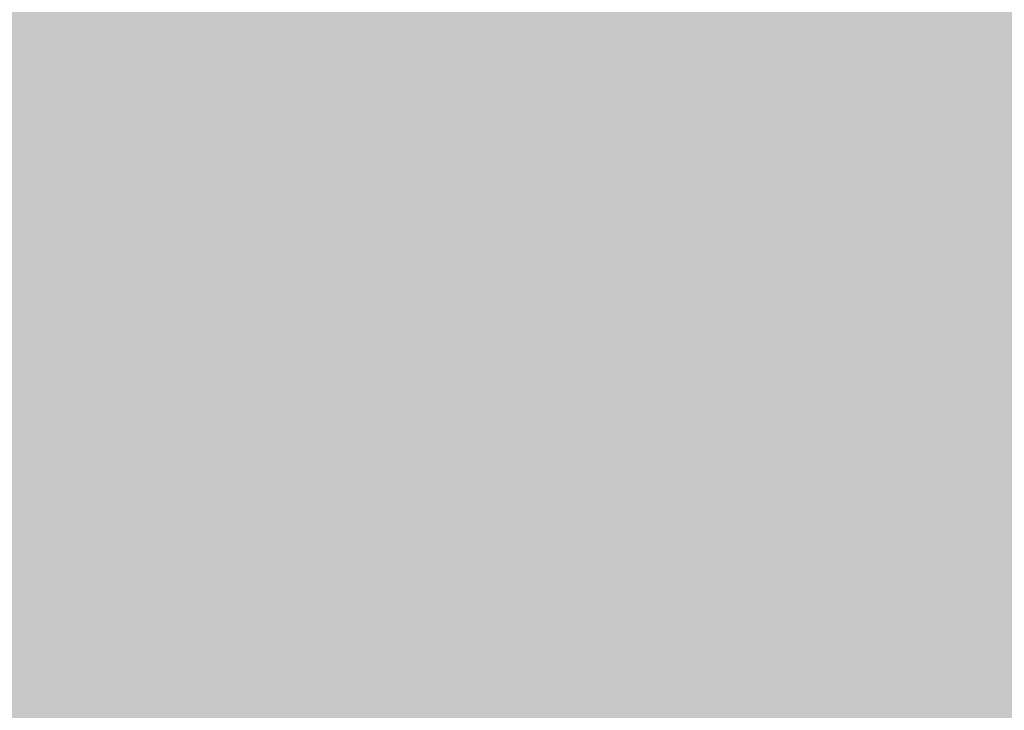
# Model space of a CAD drawing. Units: inches. Extents: x 2091 to 2899, y 967 to 2217.
# Tile 204 of 256: x 2203.18039 to 2203.25707, y 1152.30086 to 1152.35465. Entities that reach past the tile are written whole.
import ezdxf

# ---------------------------------------------------------------- set-up
doc = ezdxf.new("R2010")
doc.units = ezdxf.units.IN
doc.layers.add('A-WALL-PATT', color=141, linetype='Continuous', lineweight=13, true_color=0xadddf7)

msp = doc.modelspace()

# ---------------------------------------------------------------- hatches: boundary and pattern name
at = {"layer": 'A-WALL-PATT'}
h = msp.add_hatch(color=256, dxfattribs=at)
h.dxf.hatch_style = 1
h.paths.add_polyline_path([(2803.143603, 2050.919059), (2203.143603, 2050.919059), (2203.143603, 1090.919059), (2803.143603, 1090.919059)])
h.paths.add_polyline_path([(2635.79885, 1147.540465), (2674.524052, 1147.540465, 0.376086), (2678.529665, 1152.880202), (2678.529665, 1159.556473, 0.333335), (2674.524319, 1163.561846), (2674.524319, 1163.56185), (2674.524319, 1192.93439), (2635.805971, 1192.93439), (2597.087622, 1192.93439), (2597.087622, 1163.561846, 0.333335), (2593.082276, 1159.556473), (2593.082276, 1152.880202, 0.376086), (2597.087889, 1147.540465)], flags=0)
h.paths.add_polyline_path([(2436.010433, 1278.240778, 0.000483), (2435.952643, 1278.215027, -0.001328), (2435.935625, 1278.111693, -0.001711), (2436.11644, 1278.040758, 0.002185)], flags=0)
h.paths.add_polyline_path([(2794.143603, 1143.419059), (2794.143603, 1347.419059), (2543.370171, 1347.419059), (2543.370171, 1351.919059), (2794.143603, 1351.919059), (2794.143603, 1392.713555), (2793.947398, 1392.713555), (2793.947398, 1473.5369), (2794.143603, 1473.5369), (2794.143603, 1531.919059), (2650.143603, 1531.919059), (2650.143603, 1536.419059), (2794.143603, 1536.419059), (2794.143603, 1692.419059), (2609.375609, 1692.419059), (2609.375609, 1644.419059), (2604.875609, 1644.419059), (2604.875609, 1744.919059), (2609.375609, 1744.919059), (2609.375609, 1696.919059), (2794.143603, 1696.919059), (2794.143603, 1780.919059), (2609.643603, 1780.919059), (2493.875609, 1780.919059), (2493.875609, 1785.419059), (2609.643603, 1785.419059), (2794.143603, 1785.419059), (2794.143603, 1847.938821), (2793.951222, 1847.938821), (2793.951222, 1928.762166), (2794.143603, 1928.762166), (2794.143603, 1941.419059), (2614.143603, 1941.419059), (2614.143603, 1821.419059), (2609.643603, 1821.419059), (2609.643603, 1941.419059), (2392.143603, 1941.419059), (2392.143603, 1819.919059), (2387.643603, 1819.919059), (2387.643603, 1941.419059), (2212.143603, 1941.419059), (2212.143603, 1783.919059), (2392.143603, 1783.919059), (2392.143603, 1780.919059), (2212.143603, 1780.919059), (2212.143603, 1629.419059), (2387.643603, 1629.419059), (2387.643603, 1744.919059), (2392.143603, 1744.919059), (2392.143603, 1627.919059), (2317.143603, 1627.919059), (2317.143603, 1551.419059), (2317.143603, 1536.419059), (2459.383591, 1536.419059), (2459.383591, 1602.39648), (2463.883591, 1602.39648), (2463.883591, 1531.919059), (2456.643603, 1531.919059), (2456.643603, 1529.919059), (2452.143603, 1529.919059), (2452.143603, 1531.919059), (2312.643603, 1531.919059), (2312.643603, 1551.419059), (2306.143603, 1551.419059), (2306.143603, 1555.919059), (2308.143603, 1555.919059), (2308.143603, 1551.419059), (2312.643603, 1551.419059), (2312.643603, 1627.919059), (2212.143603, 1627.919059), (2212.143603, 1555.919059), (2270.143603, 1555.919059), (2270.143603, 1551.419059), (2212.143603, 1551.419059), (2212.143603, 1351.919059), (2272.143603, 1351.919059), (2272.143603, 1347.419059), (2212.143603, 1347.419059), (2212.143603, 1275.419059), (2308.143603, 1275.419059), (2308.143603, 1351.919059), (2452.143603, 1351.919059), (2452.143603, 1493.919059), (2456.643603, 1493.919059), (2456.643603, 1347.419059), (2312.643603, 1347.419059), (2312.643603, 1270.919059), (2212.143603, 1270.919059), (2212.143603, 1099.919059), (2281.237523, 1099.919059), (2282.871041, 1110.913803), (2282.008341, 1116.996603), (2278.557741, 1121.420403), (2268.205641, 1128.056203), (2272.087641, 1128.056203), (2273.812941, 1131.927003), (2279.420341, 1134.691903), (2285.027841, 1135.244903), (2287.615841, 1137.456803), (2288.047141, 1138.009803), (2289.341141, 1140.774703), (2291.066541, 1139.668703), (2292.360541, 1135.244903), (2295.379841, 1136.903803), (2296.242541, 1135.797903), (2297.105241, 1133.033003), (2300.124641, 1138.009803), (2303.143941, 1138.009803), (2304.437941, 1135.797903), (2303.143941, 1133.586003), (2306.594641, 1134.691903), (2307.888741, 1133.033003), (2310.908041, 1135.244903), (2313.927441, 1134.138903), (2315.62686, 1132.427102), (2308.320041, 1117.549603), (2290.203841, 1109.807903), (2288.909841, 1103.172103), (2289.272309, 1099.919059), (2434.918227, 1099.919059), (2431.593227, 1124.788059), (2429.930227, 1169.553059), (2430.927185, 1240.519694), (2435.658926, 1238.186126), (2437.135227, 1196.554059), (2438.798227, 1143.973059), (2442.678227, 1111.998059), (2446.558227, 1099.919059), (2794.143603, 1099.919059), (2794.143603, 1138.919059), (2548.032447, 1138.919059), (2548.032447, 1143.419059), (2548.032447, 1148.819059), (2546.668457, 1148.031559), (2528.685692, 1179.178622, 0.256256), (2512.032447, 1148.819059), (2512.032447, 1143.419059), (2512.032447, 1138.919059), (2507.532447, 1138.919059), (2507.532447, 1143.419059), (2507.532447, 1148.819059, 0.256256), (2490.879202, 1179.178622), (2472.896437, 1148.031559), (2471.532447, 1148.819059), (2471.532447, 1143.419059), (2467.032447, 1143.419059), (2467.032447, 1269.945786, 0.039061), (2460.909987, 1273.580059), (2467.032447, 1273.580059), (2467.032447, 1286.325364, 0.014511), (2465.216194, 1286.761905), (2467.032447, 1287.052576), (2467.032447, 1323.419059), (2471.532447, 1323.419059), (2471.532447, 1148.819059), (2489.532447, 1179.995973), (2490.896437, 1179.208473), (2490.879202, 1179.178622, -0.256256), (2507.532447, 1148.819059), (2507.532447, 1143.419059), (2512.032447, 1143.419059), (2512.032447, 1148.819059, -0.256256), (2528.685692, 1179.178622), (2528.668457, 1179.208473), (2530.032447, 1179.995973), (2548.032447, 1148.819059), (2548.032447, 1143.419059)], flags=16)
h.paths.add_polyline_path([(2607.768546, 1200.945083), (2607.768546, 1265.030625), (2597.087622, 1281.052011), (2619.784585, 1281.052011), (2627.795278, 1337.12686), (2635.79885, 1337.12686), (2643.816663, 1337.12686), (2651.827356, 1281.052011), (2674.524319, 1281.052011), (2663.843395, 1265.030625), (2663.843395, 1200.945083), (2635.805971, 1200.945083)], flags=0)
edge = h.paths.add_edge_path(flags=0)
edge.add_ellipse((13303.896215, 1272.998725), major_axis=(-10595.31304, 0.000001), ratio=0.842303870086, start_angle=0.6282372191, end_angle=0.6465540999, ccw=False)
edge.add_ellipse((2711.70045, 1156.852678), major_axis=(2.219769, 0), ratio=0.84230387, start_angle=111.535244, end_angle=180.628237, ccw=False)
edge.add_ellipse((13303.156292, 1272.998725), major_axis=(-10593.026306, 0), ratio=0.842303869544, start_angle=0.5282714718, end_angle=0.6465540971, ccw=False)
edge.add_line((2710.764596, 1175.333295), (2710.129986, 1175.333295))
edge.add_ellipse((2710.129986, 1176.579775), major_axis=(1.479846, 0), ratio=0.84230387, start_angle=180, end_angle=270, ccw=False)
edge.add_line((2708.65014, 1176.579775), (2708.65014, 1200.782914))
edge.add_ellipse((2710.129986, 1200.782914), major_axis=(1.479846, 0), ratio=0.84230387, start_angle=90, end_angle=180, ccw=False)
edge.add_line((2710.129986, 1202.029394), (2710.465075, 1202.029394))
edge.add_ellipse((13303.156292, 1272.998725), major_axis=(-10593.026306, 0), ratio=0.842303869544, start_angle=-0.0902290886, end_angle=0.3838667788, ccw=False)
edge.add_ellipse((2710.129986, 1290.927031), major_axis=(-1.479846, 0), ratio=0.84230387, start_angle=0, end_angle=90, ccw=False)
edge.add_line((2708.65014, 1290.927031), (2708.65014, 1315.13017))
edge.add_ellipse((2710.129986, 1315.13017), major_axis=(-1.479846, 0), ratio=0.84230387, start_angle=-90, end_angle=0, ccw=False)
edge.add_line((2710.129986, 1316.37665), (2710.706314, 1316.37665))
edge.add_ellipse((3238.40172, 1296.289566), major_axis=(528.234, 0), ratio=0.8423038695, start_angle=176.34957241, end_angle=177.82004969, ccw=False)
edge.add_ellipse((2775.063043, 1071.450696), major_axis=(313.307761, 0), ratio=0.8423038695, start_angle=102.12596555, end_angle=103.78052899, ccw=False)
edge.add_ellipse((2775.063043, 1078.305698), major_axis=(-305.302891, 0), ratio=0.8423038695, start_angle=-79.790461, end_angle=-77.55537271, ccw=False)
edge.add_ellipse((2695.141767, 1541.975383), major_axis=(-250.960216, 0), ratio=0.8423038695, start_angle=99.25656601, end_angle=102.55493264)
edge.add_line((2741.410326, 1334.214255), (2747.132545, 1337.378477))
edge.add_ellipse((2747.538616, 1336.857478), major_axis=(-0.739923, 0), ratio=0.8423039, start_angle=270, end_angle=307.93313, ccw=False)
edge.add_ellipse((2747.538616, 1336.857478), major_axis=(-0.739923, 0), ratio=0.8423039, start_angle=232.06687, end_angle=270, ccw=False)
edge.add_line((2747.944687, 1337.378477), (2753.666906, 1334.214255))
edge.add_ellipse((2799.935466, 1541.975383), major_axis=(250.960216, 0), ratio=0.8423038695, start_angle=257.44506736, end_angle=260.74343399)
edge.add_ellipse((2720.014189, 1078.305698), major_axis=(305.302891, 0), ratio=0.8423038695, start_angle=77.55537271, end_angle=79.790461, ccw=False)
edge.add_ellipse((2720.014189, 1071.450696), major_axis=(-313.307761, 0), ratio=0.8423038695, start_angle=256.21947101, end_angle=257.87403445, ccw=False)
edge.add_ellipse((2256.675512, 1296.289566), major_axis=(-528.234, 0), ratio=0.8423038695, start_angle=182.17995031, end_angle=183.65042759, ccw=False)
edge.add_line((2784.370918, 1316.37665), (2784.947247, 1316.37665))
edge.add_ellipse((2784.947247, 1315.13017), major_axis=(1.479846, 0), ratio=0.84230387, start_angle=0, end_angle=90, ccw=False)
edge.add_line((2786.427093, 1315.13017), (2786.427093, 1290.927031))
edge.add_ellipse((2784.947247, 1290.927031), major_axis=(1.479846, 0), ratio=0.84230387, start_angle=270, end_angle=360, ccw=False)
edge.add_ellipse((-7808.07906, 1272.998725), major_axis=(10593.026306, 0), ratio=0.842303869544, start_angle=-0.3838667788, end_angle=0.0902290886, ccw=False)
edge.add_line((2784.612157, 1202.029394), (2784.947247, 1202.029394))
edge.add_ellipse((2784.947247, 1200.782914), major_axis=(1.479846, 0), ratio=0.84230387, start_angle=0, end_angle=90, ccw=False)
edge.add_line((2786.427093, 1200.782914), (2786.427093, 1176.579775))
edge.add_ellipse((2784.947247, 1176.579775), major_axis=(-1.479846, 0), ratio=0.84230387, start_angle=90, end_angle=180, ccw=False)
edge.add_line((2784.947247, 1175.333295), (2784.312636, 1175.333295))
edge.add_ellipse((-7808.07906, 1272.998725), major_axis=(10593.026306, 0), ratio=0.842303869544, start_angle=-0.6186431963, end_angle=-0.5282714718, ccw=False)
edge.add_ellipse((2783.376783, 1156.852678), major_axis=(-2.219769, 0), ratio=0.84230387, start_angle=179.371763, end_angle=248.464757, ccw=False)
edge.add_ellipse((-7808.818983, 1272.998725), major_axis=(-10595.31304, 0.000004), ratio=0.842303865762, start_angle=179.3534459226, end_angle=179.3717628034, ccw=False)
edge.add_ellipse((2780.297303, 1153.500793), major_axis=(-5.246426, 0), ratio=0.84230387, start_angle=90, end_angle=179.353446, ccw=False)
edge.add_line((2780.297303, 1149.081708), (2714.77993, 1149.081708))
edge.add_ellipse((2714.77993, 1153.500793), major_axis=(5.246426, 0), ratio=0.84230387, start_angle=180.646554, end_angle=270, ccw=False)
edge = h.paths.add_edge_path(flags=0)
edge.add_line((2718.187367, 1151.007833), (2718.187367, 1170.472364))
edge.add_ellipse((2721.14706, 1170.472364), major_axis=(-2.959692, 0), ratio=0.84230387, start_angle=-90, end_angle=0, ccw=False)
edge.add_line((2721.14706, 1172.965324), (2773.930173, 1172.965324))
edge.add_ellipse((2773.930173, 1170.472364), major_axis=(-2.959692, 0), ratio=0.84230387, start_angle=180, end_angle=270, ccw=False)
edge.add_line((2776.889865, 1170.472364), (2776.889865, 1151.007833))
edge.add_line((2776.889865, 1151.007833), (2718.187367, 1151.007833))
edge = h.paths.add_edge_path(flags=0)
edge.add_line((2718.187367, 1180.23415), (2718.187367, 1199.057834))
edge.add_ellipse((2747.538616, 1320.39864), major_axis=(147.017924, 0), ratio=0.8423038695, start_angle=256.40186531, end_angle=283.59813469)
edge.add_line((2776.889865, 1199.057834), (2776.889865, 1180.23415))
edge.add_ellipse((2747.538616, 1301.574956), major_axis=(147.017924, 0), ratio=0.8423038695, start_angle=256.40186531, end_angle=283.59813469, ccw=False)
edge = h.paths.add_edge_path(flags=0)
edge.add_ellipse((13303.156292, 1272.998725), major_axis=(-10591.54646, 0), ratio=0.842303869555, start_angle=0.0555943135, end_angle=0.3777641939, ccw=False)
edge.add_line((2711.616859, 1262.72171), (2715.667408, 1249.495396))
edge.add_ellipse((6413.891963, 1241.691919), major_axis=(-3698.236159, 0), ratio=0.84230386955, start_angle=-0.120897369, end_angle=0.364076349)
edge.add_line((2715.761038, 1218.192455), (2711.934307, 1203.167361))
edge = h.paths.add_edge_path(flags=0)
edge.add_line((2718.187367, 1251.074566), (2716.002485, 1267.450435))
edge.add_ellipse((2742.151175, 1202.18954), major_axis=(81.772585, 0), ratio=0.84230387, start_angle=94.27742096, end_angle=111.8349538, ccw=False)
edge.add_line((2737.009748, 1270.930626), (2758.067484, 1270.930626))
edge.add_ellipse((2752.926058, 1202.18954), major_axis=(81.772585, 0), ratio=0.84230387, start_angle=68.1650462, end_angle=85.72257904, ccw=False)
edge.add_line((2779.074747, 1267.450435), (2776.889865, 1251.074566))
edge.add_ellipse((2750.338059, 1187.885356), major_axis=(79.579664, 0), ratio=0.84230387, start_angle=67.20808512, end_angle=85.1299304)
edge.add_line((2756.034656, 1254.743656), (2739.042576, 1254.743656))
edge.add_ellipse((2744.739174, 1187.885356), major_axis=(79.579664, 0), ratio=0.84230387, start_angle=94.8700696, end_angle=112.79191488)
edge = h.paths.add_edge_path(flags=0)
edge.add_line((2783.142926, 1203.167361), (2779.316194, 1218.192455))
edge.add_ellipse((-918.81473, 1241.691919), major_axis=(3698.236159, 0), ratio=0.84230386955, start_angle=-0.364076349, end_angle=0.120897369)
edge.add_line((2779.409825, 1249.495396), (2783.460373, 1262.72171))
edge.add_ellipse((-7808.07906, 1272.998725), major_axis=(-10591.54646, 0), ratio=0.84230386954, start_angle=179.6222358061, end_angle=179.9444056865, ccw=False)
edge = h.paths.add_edge_path(flags=0)
edge.add_ellipse((2734.200892, 1286.69044), major_axis=(-0.356609, 6.340078), ratio=0.60383358, start_angle=89.0020143, end_angle=253.657408, ccw=False)
edge.add_line((2730.369001, 1286.541806), (2730.369001, 1301.35198))
edge.add_line((2730.369001, 1301.35198), (2735.913311, 1305.214803))
edge.add_ellipse((2736.384917, 1304.734561), major_axis=(0.739923, 0), ratio=0.8423039, start_angle=90, end_angle=134.480211, ccw=False)
edge.add_line((2736.384917, 1305.357801), (2738.032783, 1305.357801))
edge.add_line((2738.032783, 1305.357801), (2738.032783, 1307.707927))
edge.add_ellipse((2794.201642, 1307.707927), major_axis=(56.168859, 0), ratio=0.84230387, start_angle=150.5614304, end_angle=180, ccw=False)
edge.add_ellipse((2700.875591, 1307.707927), major_axis=(-56.168859, 0), ratio=0.84230387, start_angle=180, end_angle=209.4385696, ccw=False)
edge.add_line((2757.04445, 1307.707927), (2757.04445, 1305.357801))
edge.add_line((2757.04445, 1305.357801), (2758.692316, 1305.357801))
edge.add_ellipse((2758.692316, 1304.734561), major_axis=(-0.739923, 0), ratio=0.8423039, start_angle=225.519789, end_angle=270, ccw=False)
edge.add_line((2759.163922, 1305.214803), (2764.708231, 1301.35198))
edge.add_line((2764.708231, 1301.35198), (2764.708231, 1286.541806))
edge.add_ellipse((2760.87634, 1286.69044), major_axis=(0.356609, 6.340078), ratio=0.60383358, start_angle=106.342592, end_angle=270.9979857, ccw=False)
edge.add_line((2757.04445, 1285.79709), (2757.04445, 1307.707927))
edge.add_ellipse((2700.875591, 1307.707927), major_axis=(-56.168859, 0), ratio=0.84230387, start_angle=180, end_angle=209.4385696)
edge.add_ellipse((2794.201642, 1307.707927), major_axis=(56.168859, 0), ratio=0.84230387, start_angle=150.5614304, end_angle=180)
edge.add_line((2738.032783, 1307.707927), (2738.032783, 1285.79709))
h.paths.add_polyline_path([(2417.812273, 1104.449704), (2413.492273, 1102.529704), (2410.612273, 1103.969704), (2409.172273, 1106.369704), (2407.252273, 1107.329704), (2406.292273, 1109.729704), (2405.332273, 1114.049704), (2405.332273, 1117.889704), (2406.292273, 1120.129704), (2407.252273, 1119.809704), (2408.848322, 1118.327658), (2410.173945, 1119.42417), (2410.211273, 1120.405704), (2411.040731, 1121.419054), (2410.699273, 1119.858704), (2410.173945, 1119.42417), (2410.088452, 1117.176109), (2411.132836, 1116.206324), (2413.972273, 1119.329704), (2416.852273, 1120.769704), (2416.869721, 1120.798784), (2417.035071, 1119.405116), (2417.896213, 1118.143384), (2418.292273, 1118.369704), (2419.544447, 1120.039269), (2419.360915, 1118.387487), (2419.032108, 1119.356151), (2418.398939, 1118.511926), (2419.252273, 1114.529704), (2418.794091, 1107.198795)], flags=0)
h.paths.add_polyline_path([(2508.870171, 1347.419059), (2508.370171, 1347.419059), (2508.370171, 1351.919059), (2508.870171, 1351.919059)], flags=0)
h.paths.add_polyline_path([(2473.370171, 1347.419059), (2472.370171, 1347.419059), (2467.870171, 1347.419059), (2467.870171, 1455.419059), (2472.370171, 1455.419059), (2472.370171, 1352.419059), (2473.370171, 1352.419059)], flags=0)
h.paths.add_polyline_path([(2352.106244, 1217.446197), (2349.226244, 1218.886197), (2347.786244, 1221.286197), (2345.866244, 1222.246197), (2344.906244, 1224.646197), (2343.946244, 1228.966197), (2343.946244, 1232.806197), (2344.906244, 1235.046197), (2345.866244, 1234.726197), (2347.462293, 1233.244152), (2348.787916, 1234.340663), (2348.825244, 1235.322197), (2349.654702, 1236.335547), (2349.313244, 1234.775197), (2348.787916, 1234.340663), (2348.702423, 1232.092603), (2349.746807, 1231.122817), (2352.586244, 1234.246197), (2355.466244, 1235.686197), (2355.483692, 1235.715277), (2355.649043, 1234.321609), (2356.510185, 1233.059877), (2356.906244, 1233.286197), (2358.158418, 1234.955762), (2357.974887, 1233.30398), (2357.646079, 1234.272644), (2357.012911, 1233.428419), (2357.866244, 1229.446197), (2357.408062, 1222.115288), (2356.426244, 1219.366197)], flags=0)
h.paths.add_polyline_path([(2348.2968, 1112.22442), (2347.0138, 1112.31042), (2345.5298, 1114.12742), (2345.7318, 1115.85842), (2346.8118, 1116.98242), (2346.8118, 1114.64642), (2345.8668, 1114.21442), (2346.8798, 1114.30042)], flags=0)
h.paths.add_polyline_path([(2347.0138, 1110.92642), (2346.2718, 1110.49342), (2346.6098, 1111.18642)], flags=0)
h.paths.add_polyline_path([(2345.8668, 1118.19442), (2345.5298, 1117.32942), (2343.7078, 1118.02142), (2344.3828, 1118.62642)], flags=0)
h.paths.add_polyline_path([(2346.6768, 1109.28242), (2346.0698, 1108.07142), (2345.8668, 1110.06142)], flags=0)
h.paths.add_polyline_path([(2345.0568, 1119.75142), (2343.6398, 1119.75142), (2343.9778, 1121.13542)], flags=0)
h.paths.add_polyline_path([(2345.2598, 1116.55042), (2345.1248, 1115.85842), (2344.9218, 1115.68542), (2344.7198, 1116.37742)], flags=0)
h.paths.add_polyline_path([(2345.6648, 1112.31042), (2345.4618, 1111.53242), (2344.0448, 1111.96442), (2344.6518, 1112.57042)], flags=0)
h.paths.add_polyline_path([(2345.1918, 1113.34942), (2344.4498, 1113.86842), (2344.7198, 1114.38742)], flags=0)
h.paths.add_polyline_path([(2344.6518, 1116.80942), (2344.1798, 1115.68542), (2344.6518, 1115.33942), (2343.9098, 1114.90642), (2343.0328, 1115.94442), (2343.6398, 1116.46342)], flags=0)
h.paths.add_polyline_path([(2345.8668, 1106.68642), (2344.9898, 1105.56242), (2344.5168, 1106.60042)], flags=0)
h.paths.add_polyline_path([(2344.8548, 1110.06142), (2344.5168, 1109.28242), (2344.1128, 1109.71542)], flags=0)
h.paths.add_polyline_path([(2344.0448, 1113.52242), (2343.4378, 1113.08942), (2342.7628, 1113.95442)], flags=0)
h.paths.add_polyline_path([(2344.3148, 1111.01242), (2342.9648, 1110.32042), (2342.9648, 1111.09942)], flags=0)
h.paths.add_polyline_path([(2345.1248, 1104.69742), (2344.5848, 1103.74542), (2344.4498, 1104.26442)], flags=0)
h.paths.add_polyline_path([(2342.8298, 1121.22242), (2341.7498, 1120.53042), (2340.5358, 1121.04942), (2340.1308, 1121.82842), (2340.6708, 1122.95242), (2341.1428, 1121.82842), (2341.6148, 1122.00142)], flags=0)
h.paths.add_polyline_path([(2342.9648, 1119.75142), (2343.0328, 1118.45342), (2342.0878, 1118.02142), (2342.0198, 1119.49142)], flags=0)
h.paths.add_polyline_path([(2342.6948, 1116.89642), (2341.9528, 1116.63642), (2342.0198, 1117.32942)], flags=0)
h.paths.add_polyline_path([(2343.0328, 1112.22442), (2342.0198, 1111.79142), (2341.5478, 1112.22442), (2342.3578, 1113.34942)], flags=0)
h.paths.add_polyline_path([(2343.7748, 1104.43742), (2342.6278, 1102.88042), (2342.6948, 1104.61042), (2343.4378, 1105.12942)], flags=0)
h.paths.add_polyline_path([(2342.0198, 1115.07942), (2340.8058, 1115.51242), (2340.9408, 1116.37742)], flags=0)
h.paths.add_polyline_path([(2341.4808, 1120.09742), (2341.4808, 1119.40542), (2341.0758, 1119.57842), (2341.1428, 1120.09742)], flags=0)
h.paths.add_polyline_path([(2341.8178, 1114.47342), (2340.9408, 1113.08942), (2340.8058, 1114.56042)], flags=0)
h.paths.add_polyline_path([(2341.1428, 1118.54042), (2340.9408, 1116.98242), (2339.0508, 1117.67542), (2339.0508, 1118.62642)], flags=0)
h.paths.add_polyline_path([(2342.6948, 1101.66842), (2341.9528, 1101.84142), (2342.5598, 1102.36142)], flags=0)
h.paths.add_polyline_path([(2340.3328, 1119.66542), (2338.4438, 1119.57842), (2337.9038, 1120.35742), (2339.6578, 1120.61642)], flags=0)
h.paths.add_polyline_path([(2340.3328, 1115.33942), (2340.0628, 1113.69542), (2339.3878, 1115.33942)], flags=0)
h.paths.add_polyline_path([(2341.8178, 1103.83142), (2341.5478, 1102.88042), (2341.1428, 1103.65842)], flags=0)
h.paths.add_polyline_path([(2339.0508, 1122.86642), (2337.2958, 1121.82842), (2337.0938, 1123.12542), (2337.7688, 1123.81842)], flags=0)
h.paths.add_polyline_path([(2339.1178, 1121.74142), (2338.8478, 1121.22242), (2338.1738, 1121.04942), (2338.3758, 1121.56842)], flags=0)
h.paths.add_polyline_path([(2339.1858, 1119.31942), (2338.6458, 1118.71342), (2338.2408, 1118.10742), (2338.2408, 1118.88642)], flags=0)
h.paths.add_polyline_path([(2341.1428, 1101.92842), (2340.6028, 1101.23642), (2340.0628, 1101.84142), (2340.6028, 1102.36142)], flags=0)
h.paths.add_polyline_path([(2337.6338, 1117.76142), (2336.6208, 1118.28042), (2337.2958, 1118.97242)], flags=0)
h.paths.add_polyline_path([(2336.8238, 1119.57842), (2334.7988, 1118.97242), (2335.2038, 1120.35742), (2336.5538, 1120.87642)], flags=0)
h.paths.add_polyline_path([(2339.1178, 1100.45742), (2337.3638, 1100.54342), (2336.7558, 1101.23642)], flags=0)
h.paths.add_polyline_path([(2336.3508, 1122.43342), (2336.0138, 1121.91442), (2334.9338, 1122.43342), (2334.5288, 1123.47142), (2335.7438, 1122.77942)], flags=0)
h.paths.add_polyline_path([(2334.7318, 1120.87642), (2334.2588, 1120.35742), (2334.0568, 1120.78942), (2334.5968, 1121.30842)], flags=0)
h.paths.add_polyline_path([(2334.4618, 1122.17442), (2332.5718, 1121.30842), (2331.3568, 1122.17442), (2332.0998, 1122.86642)], flags=0)
h.paths.add_polyline_path([(2334.2588, 1118.54042), (2333.3818, 1118.45342), (2333.6518, 1119.31942)], flags=0)
h.paths.add_polyline_path([(2335.5418, 1102.27442), (2334.1918, 1102.62042), (2335.2718, 1103.31242)], flags=0)
h.paths.add_polyline_path([(2332.7068, 1119.66542), (2331.6948, 1120.44342), (2332.5048, 1120.78942)], flags=0)
h.paths.add_polyline_path([(2334.7318, 1101.14942), (2333.5168, 1101.58242), (2333.9888, 1101.75542)], flags=0)
h.paths.add_polyline_path([(2332.6398, 1116.63642), (2331.0868, 1116.29042), (2331.9648, 1118.19442)], flags=0)
h.paths.add_polyline_path([(2330.7498, 1121.56842), (2330.2768, 1120.27042), (2328.5228, 1119.31942), (2328.9948, 1121.04942)], flags=0)
h.paths.add_polyline_path([(2330.7498, 1118.62642), (2330.0078, 1117.50242), (2329.8728, 1118.02142)], flags=0)
h.paths.add_polyline_path([(2332.0998, 1102.36142), (2330.5468, 1102.01442), (2331.6948, 1102.96642)], flags=0)
h.paths.add_polyline_path([(2329.5348, 1113.60842), (2329.0628, 1112.31042), (2328.5898, 1113.34942)], flags=0)
h.paths.add_polyline_path([(2328.3878, 1117.84842), (2327.5098, 1116.55042), (2327.1728, 1117.76142)], flags=0)
h.paths.add_polyline_path([(2329.7378, 1106.51342), (2329.5348, 1105.30242), (2328.2528, 1106.08142)], flags=0)
h.paths.add_polyline_path([(2328.6578, 1114.38742), (2328.0498, 1114.12742), (2328.3198, 1114.90642)], flags=0)
h.paths.add_polyline_path([(2328.3198, 1112.22442), (2327.1058, 1112.13742), (2326.7008, 1112.65642)], flags=0)
h.paths.add_polyline_path([(2326.9028, 1115.25242), (2326.7008, 1114.12742), (2325.2158, 1113.60842), (2326.0928, 1115.33942)], flags=0)
h.paths.add_polyline_path([(2326.6328, 1108.33042), (2326.0928, 1107.37942), (2325.8908, 1108.50342), (2326.4978, 1109.10942)], flags=0)
h.paths.add_polyline_path([(2615.143603, 1531.919059), (2609.643603, 1531.919059), (2609.643603, 1620.419059), (2614.143603, 1620.419059), (2614.143603, 1536.419059), (2615.143603, 1536.419059)], flags=0)
h.paths.add_polyline_path([(2545.143603, 1563.419059), (2464.143603, 1563.419059), (2464.143603, 1632.419059), (2509.143603, 1632.419059), (2509.143603, 1627.919059), (2509.143603, 1603.919059), (2468.643603, 1603.919059), (2468.643603, 1567.919059), (2540.643603, 1567.919059), (2540.643603, 1591.919059), (2545.143603, 1591.919059)], flags=0)
h.paths.add_polyline_path([(2388.969048, 1549.985735), (2357.434181, 1549.985735), (2357.434181, 1623.360778), (2399.362777, 1623.360778), (2435.689465, 1623.360778), (2435.592547, 1602.559273), (2435.592547, 1602.39648), (2388.969048, 1602.39648)], flags=0)
h.paths.add_polyline_path([(2388.880628, 1555.809151), (2374.904429, 1555.809151), (2374.904429, 1600.571564), (2374.904429, 1615.457645), (2406.350877, 1615.457645), (2406.350877, 1618.939431), (2412.174293, 1615.457645), (2406.350877, 1611.97586), (2406.350877, 1615.457645), (2388.880628, 1615.457645)], flags=0)
h.paths.add_polyline_path([(2568.875609, 1644.419059), (2453.375609, 1644.419059), (2453.375609, 1785.419059), (2457.875609, 1785.419059), (2457.875609, 1648.919059), (2568.875609, 1648.919059)], flags=0)
h.paths.add_polyline_path([(2212.143603, 1945.919059), (2212.143603, 2041.919059), (2794.143603, 2041.919059), (2794.143603, 1945.919059)], flags=16)
h.paths.add_polyline_path([(2271.082728, 1964.317238), (2776.852968, 1964.317238), (2776.852968, 2037.169623), (2271.082728, 2037.169623)], flags=8)
h.paths.add_polyline_path([(2380.649285, 1536.824144), (2461.040809, 1536.824144), (2461.040809, 1554.652587), (2380.649285, 1554.652587)], flags=8)
h.paths.add_polyline_path([(2240.755709, 1609.725451), (2309.185829, 1609.725451), (2309.185829, 1617.698204), (2240.755709, 1617.698204)], flags=8)
h.paths.add_polyline_path([(2212.677255, 1313.504102), (2282.59152, 1313.504102), (2282.59152, 1322.745239), (2212.677255, 1322.745239)], flags=8)
h.paths.add_polyline_path([(2457.111976, 1114.778574), (2558.481581, 1114.778574), (2558.481581, 1142.219682), (2457.111976, 1142.219682)], flags=8)
h.paths.add_polyline_path([(2473.442337, 1273.010067), (2604.641226, 1273.010067), (2604.641226, 1318.346935), (2473.442337, 1318.346935)], flags=8)
h.paths.add_polyline_path([(2638.876302, 1626.977432), (2684.250367, 1627.976738), (2684.038483, 1637.597494), (2638.664417, 1636.598188)], flags=8)
h.paths.add_polyline_path([(2537.590554, 1453.793447), (2628.389547, 1453.793447), (2628.389547, 1475.344811), (2537.590554, 1475.344811)], flags=8)
h.paths.add_polyline_path([(2504.137638, 1714.632397), (2554.647187, 1714.632397), (2554.647187, 1730.237712), (2504.137638, 1730.237712)], flags=8)
h.paths.add_polyline_path([(2487.501181, 1575.651872), (2535.097121, 1575.651872), (2535.097121, 1598.377646), (2487.501181, 1598.377646)], flags=8)
h.paths.add_polyline_path([(2709.0994, 1735.710278), (2740.016601, 1735.710278), (2740.016601, 1749.937641), (2709.0994, 1749.937641)], flags=8)
h.paths.add_polyline_path([(2442.438424, 1792.171657), (2564.728835, 1792.171657), (2564.728835, 1842.000163), (2442.438424, 1842.000163)], flags=8)
h.paths.add_polyline_path([(2655.815801, 1809.644076), (2789.520142, 1806.693796), (2790.084977, 1832.291638), (2656.380635, 1835.241918)], flags=8)
h.paths.add_polyline_path([(2234.842697, 1797.720143), (2368.592851, 1794.768852), (2369.160718, 1820.504132), (2235.410564, 1823.455423)], flags=8)
h.paths.add_polyline_path([(2245.138466, 1644.006335), (2398.427733, 1640.6239), (2398.994842, 1666.32482), (2245.705575, 1669.707255)], flags=8)
h.paths.add_polyline_path([(2306.142847, 1431.168519), (2413.768314, 1428.793687), (2414.333148, 1454.391529), (2306.707682, 1456.76636)], flags=8)
h.paths.add_polyline_path([(2306.834582, 1458.233145), (2393.380484, 1456.323449), (2393.932808, 1481.354358), (2307.386907, 1483.264054)], flags=8)

doc.saveas('drawing.dxf')
